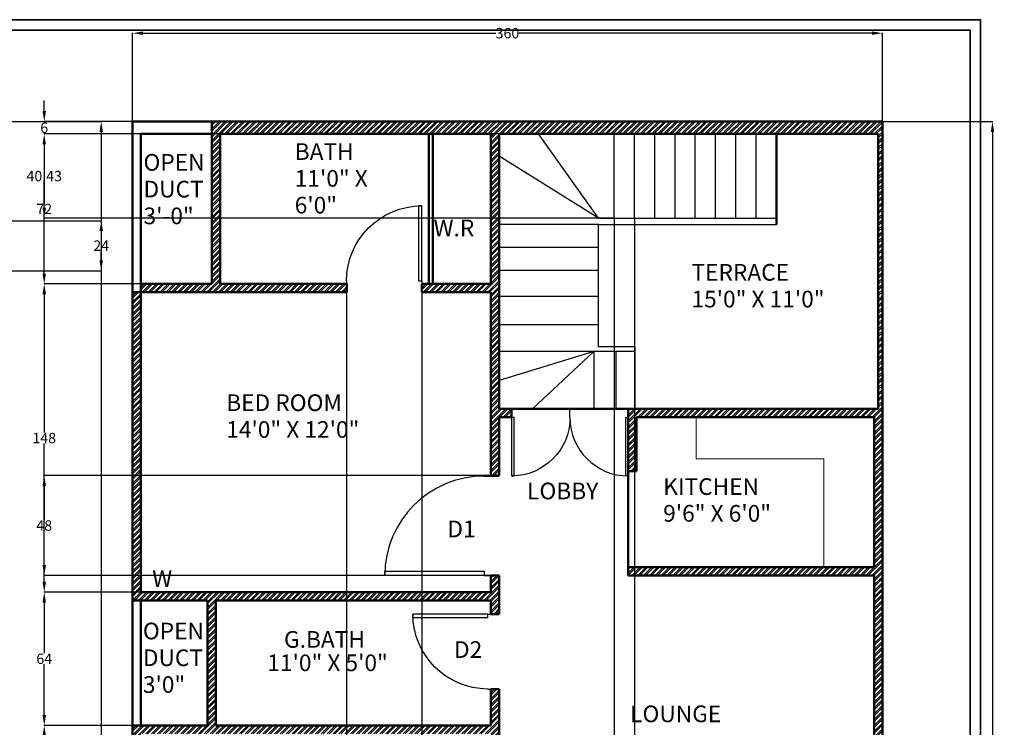
# Model space of a CAD drawing. Units: inches. Extents: x -35 to 905, y -602 to 298.
# Tile 4 of 4: x 429 to 902, y -42 to 298. Entities that reach past the tile are written whole.
import ezdxf

# ---------------------------------------------------------------- set-up
doc = ezdxf.new("R2010")
doc.units = ezdxf.units.IN
doc.header["$MEASUREMENT"] = 0
for name, color, linetype, lineweight in [('A-ANNO-DIMS', 2, 'Continuous', 18), ('A-ANNO-TEXT', 3, 'Continuous', 18), ('A-ANNO-TTLB', 7, 'Continuous', 35), ('A-AREA-IDEN', 7, 'Continuous', 18), ('A-DOOR', 4, 'Continuous', 25), ('A-FLOR-FIXT', 8, 'Continuous', 18), ('A-FLOR-STRS', 3, 'Continuous', 25), ('A-WALL', 7, 'Continuous', 50), ('A-WALL-PATT', 8, 'Continuous', 13)]:
    doc.layers.add(name, color=color, linetype=linetype, lineweight=lineweight)
doc.styles.get("Standard").update_dxf_attribs({"font": 'arial.ttf'})
doc.dimstyles.get("Standard").update_dxf_attribs({"dimtxt": 5, "dimasz": 5, "dimexe": 0.18, "dimexo": 0.0625, "dimgap": 0.09, "dimtad": 0, "dimtih": 1, "dimtoh": 1, "dimdec": 1, "dimzin": 0, "dimdsep": 46, "dimlunit": 4, "dimtxsty": 'Standard', "dimcen": 0.09, "dimadec": 0, "dimazin": 0, "dimtfac": 1, "dimtdec": 1, "dimtofl": 0, "dimtmove": 0, "dimatfit": 3, "dimfxl": 1, "dimtolj": 1, "dimtzin": 0, "dimarcsym": 0})

# ---------------------------------------------------------------- blocks, each defined once
blk = doc.blocks.new('*U2')
for p, q in [((0, 0), (0, -6)), ((40, 0), (40, -6))]:
    blk.add_line(p, q)
blk.add_lwpolyline([(0, 0), (0, 40), (1.75, 40), (1.75, 0)], close=True)
blk.add_arc((0, 0), 40, 0, 90)
blk = doc.blocks.new('*D18')
at = {"layer": 'A-ANNO-DIMS', "color": 0, "lineweight": -2, "ltscale": 0.3, "transparency": 16777216}
for p, q in [((377.85, 249.35), (468.36, 249.35)), ((468.18, 244.35), (468.18, -104.51)), ((468.18, -458.65), (468.18, -109.8)), ((377.85, -463.65), (468.36, -463.65))]:
    blk.add_line(p, q, dxfattribs=at)
at = {"layer": 'A-ANNO-DIMS', "color": 0, "ltscale": 0.3, "transparency": 16777216}
for points in [[(467.35, 244.35), (469.02, 244.35), (468.18, 249.35)], [(467.35, -458.65), (469.02, -458.65), (468.18, -463.65)]]:
    blk.add_solid(points, dxfattribs=at)
at = {"layer": 'Defpoints', "color": 0, "ltscale": 0.3, "transparency": 16777216}
for p in [(377.78, 249.35), (377.78, -463.65), (468.18, -463.65)]:
    blk.add_point(p, dxfattribs=at)
at = {"layer": 'A-ANNO-DIMS', "color": 0, "ltscale": 0.3, "transparency": 16777216, "insert": (468.18, -107.15), "char_height": 5, "attachment_point": 5}
blk.add_mtext('\\A1;713', dxfattribs=at)
blk = doc.blocks.new('*D23')
at = {"layer": 'A-ANNO-DIMS', "color": 0, "lineweight": -2, "ltscale": 0.3, "transparency": 16777216}
for p, q in [((101.85, 201.71), (468.36, 201.71)), ((468.18, 196.71), (468.18, 192.31)), ((468.18, 182.71), (468.18, 187.11)), ((101.85, 177.71), (468.36, 177.71))]:
    blk.add_line(p, q, dxfattribs=at)
at = {"layer": 'A-ANNO-DIMS', "color": 0, "ltscale": 0.3, "transparency": 16777216}
for points in [[(467.35, 196.71), (469.02, 196.71), (468.18, 201.71)], [(467.35, 182.71), (469.02, 182.71), (468.18, 177.71)]]:
    blk.add_solid(points, dxfattribs=at)
at = {"layer": 'Defpoints', "color": 0, "ltscale": 0.3, "transparency": 16777216}
for p in [(101.78, 201.71), (468.18, 201.71), (101.78, 177.71)]:
    blk.add_point(p, dxfattribs=at)
at = {"layer": 'A-ANNO-DIMS', "color": 0, "ltscale": 0.3, "transparency": 16777216, "insert": (468.18, 189.71), "char_height": 5, "attachment_point": 5}
blk.add_mtext('\\A1;24', dxfattribs=at)
blk = doc.blocks.new('*D31')
at = {"layer": 'A-ANNO-DIMS', "color": 0, "lineweight": -2, "ltscale": 0.3, "transparency": 16777216}
for p, q in [((483.24, 249.41), (483.24, 291.93)), ((488.24, 291.75), (657.64, 291.75)), ((838.24, 291.75), (668.84, 291.75)), ((843.24, 249.41), (843.24, 291.93))]:
    blk.add_line(p, q, dxfattribs=at)
at = {"layer": 'A-ANNO-DIMS', "color": 0, "ltscale": 0.3, "transparency": 16777216}
for points in [[(488.24, 292.58), (488.24, 290.91), (483.24, 291.75)], [(838.24, 292.58), (838.24, 290.91), (843.24, 291.75)]]:
    blk.add_solid(points, dxfattribs=at)
at = {"layer": 'Defpoints', "color": 0, "ltscale": 0.3, "transparency": 16777216}
for p in [(843.24, 291.75), (483.24, 249.35), (843.24, 249.35)]:
    blk.add_point(p, dxfattribs=at)
at = {"layer": 'A-ANNO-DIMS', "color": 0, "ltscale": 0.3, "transparency": 16777216, "insert": (663.24, 291.75), "char_height": 5, "attachment_point": 5}
blk.add_mtext('\\A1;360', dxfattribs=at)
blk = doc.blocks.new('*D32')
at = {"layer": 'A-ANNO-DIMS', "color": 0, "lineweight": -2, "ltscale": 0.3, "transparency": 16777216}
for p, q in [((440.84, 254.35), (440.84, 259.35)), ((483.18, 249.35), (440.66, 249.35)), ((487.18, 243.35), (440.66, 243.35)), ((440.84, 238.35), (440.84, 233.35))]:
    blk.add_line(p, q, dxfattribs=at)
at = {"layer": 'A-ANNO-DIMS', "color": 0, "ltscale": 0.3, "transparency": 16777216}
for points in [[(440.01, 254.35), (441.67, 254.35), (440.84, 249.35)], [(440.01, 238.35), (441.67, 238.35), (440.84, 243.35)]]:
    blk.add_solid(points, dxfattribs=at)
at = {"layer": 'Defpoints', "color": 0, "ltscale": 0.3, "transparency": 16777216}
for p in [(483.24, 249.35), (440.84, 243.35), (487.24, 243.35)]:
    blk.add_point(p, dxfattribs=at)
at = {"layer": 'A-ANNO-DIMS', "color": 0, "ltscale": 0.3, "transparency": 16777216, "insert": (440.84, 246.35), "char_height": 5, "attachment_point": 5}
blk.add_mtext('\\A1;6', dxfattribs=at)
blk = doc.blocks.new('*D33')
at = {"layer": 'A-ANNO-DIMS', "color": 0, "lineweight": -2, "ltscale": 0.3, "transparency": 16777216}
for p, q in [((487.18, 243.35), (440.66, 243.35)), ((440.84, 238.35), (440.84, 209.95)), ((440.84, 176.35), (440.84, 204.75)), ((487.18, 171.35), (440.66, 171.35))]:
    blk.add_line(p, q, dxfattribs=at)
at = {"layer": 'A-ANNO-DIMS', "color": 0, "ltscale": 0.3, "transparency": 16777216}
for points in [[(440.01, 238.35), (441.67, 238.35), (440.84, 243.35)], [(440.01, 176.35), (441.67, 176.35), (440.84, 171.35)]]:
    blk.add_solid(points, dxfattribs=at)
at = {"layer": 'Defpoints', "color": 0, "ltscale": 0.3, "transparency": 16777216}
for p in [(487.24, 243.35), (440.84, 171.35), (487.24, 171.35)]:
    blk.add_point(p, dxfattribs=at)
at = {"layer": 'A-ANNO-DIMS', "color": 0, "ltscale": 0.3, "transparency": 16777216, "insert": (440.84, 207.35), "char_height": 5, "attachment_point": 5}
blk.add_mtext('\\A1;72', dxfattribs=at)
blk = doc.blocks.new('*D34')
at = {"layer": 'A-ANNO-DIMS', "color": 0, "lineweight": -2, "ltscale": 0.3, "transparency": 16777216}
for p, q in [((487.18, 171.35), (440.66, 171.35)), ((440.84, 166.35), (440.84, 99.99)), ((440.84, 28.35), (440.84, 94.7)), ((487.18, 23.35), (440.66, 23.35))]:
    blk.add_line(p, q, dxfattribs=at)
at = {"layer": 'A-ANNO-DIMS', "color": 0, "ltscale": 0.3, "transparency": 16777216}
for points in [[(440.01, 166.35), (441.67, 166.35), (440.84, 171.35)], [(440.01, 28.35), (441.67, 28.35), (440.84, 23.35)]]:
    blk.add_solid(points, dxfattribs=at)
at = {"layer": 'Defpoints', "color": 0, "ltscale": 0.3, "transparency": 16777216}
for p in [(487.24, 171.35), (440.84, 23.35), (487.24, 23.35)]:
    blk.add_point(p, dxfattribs=at)
at = {"layer": 'A-ANNO-DIMS', "color": 0, "ltscale": 0.3, "transparency": 16777216, "insert": (440.84, 97.35), "char_height": 5, "attachment_point": 5}
blk.add_mtext('\\A1;148', dxfattribs=at)
blk = doc.blocks.new('*D35')
at = {"layer": 'A-ANNO-DIMS', "color": 0, "lineweight": -2, "ltscale": 0.3, "transparency": 16777216}
for p, q in [((487.18, 23.35), (440.66, 23.35)), ((440.84, 18.35), (440.84, -6.01)), ((440.84, -35.65), (440.84, -11.3)), ((487.18, -40.65), (440.66, -40.65))]:
    blk.add_line(p, q, dxfattribs=at)
at = {"layer": 'A-ANNO-DIMS', "color": 0, "ltscale": 0.3, "transparency": 16777216}
for points in [[(440.01, 18.35), (441.67, 18.35), (440.84, 23.35)], [(440.01, -35.65), (441.67, -35.65), (440.84, -40.65)]]:
    blk.add_solid(points, dxfattribs=at)
at = {"layer": 'Defpoints', "color": 0, "ltscale": 0.3, "transparency": 16777216}
for p in [(487.24, 23.35), (440.84, -40.65), (487.24, -40.65)]:
    blk.add_point(p, dxfattribs=at)
at = {"layer": 'A-ANNO-DIMS', "color": 0, "ltscale": 0.3, "transparency": 16777216, "insert": (440.84, -8.65), "char_height": 5, "attachment_point": 5}
blk.add_mtext('\\A1;64', dxfattribs=at)
blk = doc.blocks.new('*D36')
at = {"layer": 'A-ANNO-DIMS', "color": 0, "lineweight": -2, "ltscale": 0.3, "transparency": 16777216}
for p, q in [((487.18, -40.65), (440.66, -40.65)), ((440.84, -45.65), (440.84, -112.01)), ((440.84, -183.65), (440.84, -117.3)), ((487.18, -188.65), (440.66, -188.65))]:
    blk.add_line(p, q, dxfattribs=at)
at = {"layer": 'A-ANNO-DIMS', "color": 0, "ltscale": 0.3, "transparency": 16777216}
for points in [[(440.01, -45.65), (441.67, -45.65), (440.84, -40.65)], [(440.01, -183.65), (441.67, -183.65), (440.84, -188.65)]]:
    blk.add_solid(points, dxfattribs=at)
at = {"layer": 'Defpoints', "color": 0, "ltscale": 0.3, "transparency": 16777216}
for p in [(487.24, -40.65), (440.84, -188.65), (487.24, -188.65)]:
    blk.add_point(p, dxfattribs=at)
at = {"layer": 'A-ANNO-DIMS', "color": 0, "ltscale": 0.3, "transparency": 16777216, "insert": (440.84, -114.65), "char_height": 5, "attachment_point": 5}
blk.add_mtext('\\A1;148', dxfattribs=at)
blk = doc.blocks.new('*D40')
at = {"layer": 'A-ANNO-DIMS', "color": 0, "lineweight": -2, "ltscale": 0.3, "transparency": 16777216}
for p, q in [((843.3, 249.35), (896.28, 249.35)), ((896.1, 244.35), (896.1, -104.51)), ((896.1, -458.65), (896.1, -109.8)), ((843.3, -463.65), (896.28, -463.65))]:
    blk.add_line(p, q, dxfattribs=at)
at = {"layer": 'A-ANNO-DIMS', "color": 0, "ltscale": 0.3, "transparency": 16777216}
for points in [[(895.27, 244.35), (896.94, 244.35), (896.1, 249.35)], [(895.27, -458.65), (896.94, -458.65), (896.1, -463.65)]]:
    blk.add_solid(points, dxfattribs=at)
at = {"layer": 'Defpoints', "color": 0, "ltscale": 0.3, "transparency": 16777216}
for p in [(843.24, 249.35), (843.24, -463.65), (896.1, -463.65)]:
    blk.add_point(p, dxfattribs=at)
at = {"layer": 'A-ANNO-DIMS', "color": 0, "ltscale": 0.3, "transparency": 16777216, "insert": (896.1, -107.15), "char_height": 5, "attachment_point": 5}
blk.add_mtext('\\A1;713', dxfattribs=at)
blk = doc.blocks.new('*D48')
at = {"layer": 'A-ANNO-DIMS', "color": 0, "lineweight": -2, "ltscale": 0.3, "transparency": 16777216}
for p, q in [((585.99, 167.28), (585.99, -506.23)), ((622.06, 167.28), (622.06, -506.23)), ((590.99, -506.05), (593.54, -506.05)), ((617.06, -506.05), (614.51, -506.05))]:
    blk.add_line(p, q, dxfattribs=at)
at = {"layer": 'A-ANNO-DIMS', "color": 0, "ltscale": 0.3, "transparency": 16777216}
for points in [[(590.99, -505.22), (590.99, -506.89), (585.99, -506.05)], [(617.06, -505.22), (617.06, -506.89), (622.06, -506.05)]]:
    blk.add_solid(points, dxfattribs=at)
at = {"layer": 'Defpoints', "color": 0, "ltscale": 0.3, "transparency": 16777216}
for p in [(585.99, 167.35), (622.06, 167.35), (622.06, -506.05)]:
    blk.add_point(p, dxfattribs=at)
at = {"layer": 'A-ANNO-DIMS', "color": 0, "ltscale": 0.3, "transparency": 16777216, "insert": (604.02, -506.05), "char_height": 5, "attachment_point": 5}
blk.add_mtext('\\A1;36.065', dxfattribs=at)
blk = doc.blocks.new('*D51')
at = {"layer": 'A-ANNO-DIMS', "color": 0, "lineweight": -2, "ltscale": 0.3, "transparency": 16777216}
for p, q in [((655.18, 79.35), (440.66, 79.35)), ((440.84, 74.35), (440.84, 57.99)), ((440.84, 36.35), (440.84, 52.7)), ((655.18, 31.35), (440.66, 31.35))]:
    blk.add_line(p, q, dxfattribs=at)
at = {"layer": 'A-ANNO-DIMS', "color": 0, "ltscale": 0.3, "transparency": 16777216}
for points in [[(440.01, 74.35), (441.67, 74.35), (440.84, 79.35)], [(440.01, 36.35), (441.67, 36.35), (440.84, 31.35)]]:
    blk.add_solid(points, dxfattribs=at)
at = {"layer": 'Defpoints', "color": 0, "ltscale": 0.3, "transparency": 16777216}
for p in [(440.84, 79.35), (655.24, 79.35), (655.24, 31.35)]:
    blk.add_point(p, dxfattribs=at)
at = {"layer": 'A-ANNO-DIMS', "color": 0, "ltscale": 0.3, "transparency": 16777216, "insert": (440.84, 55.35), "char_height": 5, "attachment_point": 5}
blk.add_mtext('\\A1;48', dxfattribs=at)
blk = doc.blocks.new('*D52')
at = {"layer": 'A-ANNO-DIMS', "color": 0, "lineweight": -2, "ltscale": 0.3, "transparency": 16777216}
for p, q in [((714.42, 202.86), (714.42, -506.23)), ((724.17, 202.86), (724.17, -506.23)), ((709.42, -506.05), (704.42, -506.05)), ((729.17, -506.05), (734.17, -506.05))]:
    blk.add_line(p, q, dxfattribs=at)
at = {"layer": 'A-ANNO-DIMS', "color": 0, "ltscale": 0.3, "transparency": 16777216}
for points in [[(709.42, -505.22), (709.42, -506.89), (714.42, -506.05)], [(729.17, -505.22), (729.17, -506.89), (724.17, -506.05)]]:
    blk.add_solid(points, dxfattribs=at)
at = {"layer": 'Defpoints', "color": 0, "ltscale": 0.3, "transparency": 16777216}
for p in [(714.42, 202.92), (724.17, 202.92), (724.17, -506.05)]:
    blk.add_point(p, dxfattribs=at)
at = {"layer": 'A-ANNO-DIMS', "color": 0, "ltscale": 0.3, "transparency": 16777216, "insert": (742.7, -506.05), "char_height": 5, "attachment_point": 5}
blk.add_mtext('\\A1;9.753', dxfattribs=at)
blk = doc.blocks.new('*D53')
at = {"layer": 'A-ANNO-DIMS', "color": 0, "lineweight": -2, "ltscale": 0.3, "transparency": 16777216}
for p, q in [((714.36, 243.35), (440.66, 243.35)), ((440.84, 238.35), (440.84, 225.78)), ((440.84, 207.92), (440.84, 220.49)), ((714.36, 202.92), (440.66, 202.92))]:
    blk.add_line(p, q, dxfattribs=at)
at = {"layer": 'A-ANNO-DIMS', "color": 0, "ltscale": 0.3, "transparency": 16777216}
for points in [[(440.01, 238.35), (441.67, 238.35), (440.84, 243.35)], [(440.01, 207.92), (441.67, 207.92), (440.84, 202.92)]]:
    blk.add_solid(points, dxfattribs=at)
at = {"layer": 'Defpoints', "color": 0, "ltscale": 0.3, "transparency": 16777216}
for p in [(714.42, 243.35), (440.84, 202.92), (714.42, 202.92)]:
    blk.add_point(p, dxfattribs=at)
at = {"layer": 'A-ANNO-DIMS', "color": 0, "ltscale": 0.3, "transparency": 16777216, "insert": (440.84, 223.13), "char_height": 5, "attachment_point": 5}
blk.add_mtext('\\A1;40.43', dxfattribs=at)

msp = doc.modelspace()

# ---------------------------------------------------------------- hatches: boundary and pattern name
at = {"layer": 'A-WALL-PATT', "ltscale": 0.3}
h = msp.add_hatch(dxfattribs=at)
h.set_pattern_fill('ANSI32', color=256, scale=5.3)
h.set_pattern_definition([(45, (-58.8752, 0), (-1.4053747, 1.4053747), []), (45, (-57.9383, 0), (-1.4053747, 1.4053747), [])])
h.paths.add_polyline_path([(843.2385, 107.3466), (843.2385, 249.3466), (521.2385, 249.3466), (521.2385, 171.3466), (487.2385, 171.3466), (487.2385, 167.3466), (586.0557, 167.3466), (586.0557, 171.3466), (567.2385, 171.3466), (525.2385, 171.3466), (525.2385, 243.3466), (571.2385, 243.3466), (655.2385, 243.3466), (655.2385, 213.7106), (655.2385, 171.3466), (622.0557, 171.3466), (622.0557, 167.3466), (655.2385, 167.3466), (655.2385, 79.3466), (659.2385, 79.3466), (659.2385, 107.3466), (665.2408, 107.3466), (665.2408, 111.3466), (659.2385, 111.3466), (659.2385, 213.7106), (659.2385, 243.3466), (841.2385, 243.3466), (841.2385, 111.3466), (721.2578, 111.3466), (721.2578, 107.1453), (721.2578, 81.4115), (725.2385, 81.4115), (725.2385, 107.3466), (839.2385, 107.3466), (839.2385, 35.3466), (721.2385, 35.3466), (721.2385, 31.3466), (839.2385, 31.3466), (839.2385, -160.6534), (713.2385, -160.6534), (713.2385, -164.6534), (713.2385, -212.6534), (717.2385, -212.6534), (717.2385, -164.6534), (843.2385, -164.6534), (849.7023, -164.6534), (849.7023, -260.6534), (843.2385, -260.6534), (843.2385, -264.6534), (853.7023, -264.6534), (853.7023, -160.6534), (843.2385, -160.6534)])
h.paths.add_polyline_path([(655.2385, -188.6534), (655.2385, -192.6534), (659.2385, -192.6534), (659.2385, -23.1851), (655.2385, -23.1851), (655.2385, -40.6534), (523.2385, -40.6534), (523.2385, 19.3466), (655.2385, 19.3466), (655.2385, 12.8149), (659.2385, 12.8149), (659.2385, 31.3466), (655.2385, 31.3466), (655.2385, 23.3466), (487.2385, 23.3466), (487.2385, 167.3466), (483.2385, 167.3466), (483.2385, 19.3466), (519.2385, 19.3466), (519.2385, -40.6534), (483.2385, -40.6534), (483.2385, -463.6534), (487.2385, -463.6534), (487.2385, -422.6534), (496.4926, -422.6534), (496.4926, -422.2505), (496.4926, -418.6534), (487.2385, -418.6534), (487.2385, -315.6534), (487.2385, -192.6534), (487.2385, -44.6534), (655.2385, -44.6534)])
h.paths.add_polyline_path([(523.2385, -315.6534), (568.9907, -315.6534), (568.9907, -311.6534), (527.2385, -311.6534), (527.2385, -254.1534), (608.2385, -254.1534), (608.2385, -311.6534), (604.9907, -311.6534), (604.9907, -315.6534), (612.2385, -315.6534), (612.2385, -250.1534), (612.2385, -188.6534), (604.9907, -188.6534), (604.9907, -192.6534), (608.2385, -192.6534), (608.2385, -250.1534), (527.2385, -250.1534), (527.2385, -192.6534), (568.8266, -192.6534), (568.8266, -188.6534), (523.2385, -188.6534)], flags=17)
h.paths.add_polyline_path([(655.2385, -313.832), (655.2385, -418.6534), (520.4926, -418.6534), (520.4926, -422.6534), (655.2385, -422.6534), (655.2385, -461.6534), (655.2385, -463.6534), (659.2385, -463.6534), (659.2385, -457.6052), (659.2385, -422.6534), (664.6743, -422.6534), (664.6743, -422.2478), (664.6743, -418.6534), (659.2385, -418.6534), (659.2385, -311.6534), (669.6291, -302.6097), (667.0409, -299.5595), (655.2385, -309.832), (649.2787, -309.832), (649.2787, -313.832)])
h.paths.add_polyline_path([(839.2385, -264.6534), (839.2385, -407.6534), (836.0142, -407.6534), (836.0142, -411.6534), (839.2385, -411.6534), (839.2385, -459.6534), (767.2385, -459.6534), (767.2385, -411.6534), (800.0142, -411.6534), (800.0142, -407.6534), (767.2385, -407.6534), (763.2385, -407.6534), (763.2385, -418.6534), (688.6743, -418.6534), (688.6743, -422.6534), (763.2385, -422.6534), (763.2385, -463.6534), (843.2385, -463.6534), (843.2385, -260.6534), (715.7415, -260.6534), (715.7415, -251.2468), (711.7415, -251.2468), (711.7415, -260.6534), (704.4179, -267.0277), (702.7449, -268.4838), (705.371, -271.5011), (707.044, -270.0449), (713.2385, -264.6534)])
h.paths.add_polyline_path([(592.7587, -420.6534), (607.3071, -420.6534), (607.3071, -408.6534), (592.7587, -408.6534)], flags=24)
h.paths.add_polyline_path([(723.9564, -420.6534), (738.5048, -420.6534), (738.5048, -408.6534), (723.9564, -408.6534)], flags=24)

# ---------------------------------------------------------------- linework, layer by layer
at = {"layer": 'A-ANNO-TTLB', "ltscale": 0.3}
for points in [[(-16.7606, 298.2205), (890.3824, 298.2205), (890.3824, -602.0527), (-16.7606, -602.0527)], [(-11.7606, 293.2205), (885.3824, 293.2205), (885.3824, -599.6301), (-11.7606, -599.6301)]]:
    msp.add_lwpolyline(points, close=True, dxfattribs=at)
at = {"layer": 'A-FLOR-FIXT', "ltscale": 0.3}
for p, q in [((753.8854, 87.3211), (753.8854, 107.3466)), ((815.1608, 87.3211), (753.8854, 87.3211)), ((815.1608, 81.4115), (815.1608, 87.3211))]:
    msp.add_line(p, q, dxfattribs=at)
at = {"layer": 'A-FLOR-FIXT'}
msp.add_line((815.1608, 81.4115), (815.1608, 35.3466), dxfattribs=at)
at = {"layer": 'A-FLOR-STRS', "ltscale": 0.3}
for p, q in [((706.8936, 202.9184), (678.1479, 243.3466)), ((714.4218, 202.9184), (714.4218, 243.3466)), ((724.1748, 202.9184), (724.1748, 243.3466)), ((733.9277, 202.9184), (733.9277, 243.3466)), ((743.6806, 202.9184), (743.6806, 243.3466)), ((753.4336, 202.9184), (753.4336, 243.3466)), ((763.1865, 202.9184), (763.1865, 243.3466)), ((772.9394, 202.9184), (772.9394, 243.3466)), ((782.6924, 202.9184), (782.6924, 243.3466)), ((706.8936, 202.9184), (659.2385, 232.7531)), ((706.8936, 199.9184), (659.2385, 199.9184)), ((706.8936, 202.9184), (792.4453, 202.9184)), ((706.8936, 141.0839), (706.8936, 199.9184)), ((706.8936, 199.9184), (792.4453, 199.9184)), ((706.8936, 188.8347), (659.2385, 188.8347)), ((706.8936, 177.8594), (659.2385, 177.8594)), ((706.8936, 165.2442), (659.2385, 165.2442)), ((706.8936, 151.7806), (659.2385, 151.7806)), ((724.4958, 138.8376), (659.2385, 138.8376)), ((704.7572, 138.8376), (659.2385, 124.9608)), ((704.7572, 138.8376), (675.2188, 111.3466)), ((704.7572, 138.8376), (704.7572, 111.3466)), ((724.4958, 141.0839), (706.8936, 141.0839)), ((715.2345, 138.8376), (715.2345, 111.3466)), ((724.4958, 111.3466), (724.4958, 141.0839)), ((721.2385, 111.3466), (724.4958, 111.3466))]:
    msp.add_line(p, q, dxfattribs=at)
at = {"layer": 'A-WALL'}
for p, q in [((483.2385, 249.3466), (483.2385, -463.6534)), ((483.2385, 249.3466), (843.2385, 249.3466)), ((521.2385, 249.3466), (521.2385, 171.3466)), ((843.2385, 249.3466), (843.2385, 107.3466)), ((487.2385, 243.3466), (487.2385, 167.3466)), ((487.2385, 243.3466), (521.2385, 243.3466)), ((525.2385, 243.3466), (525.2385, 171.3466)), ((525.2385, 243.3466), (571.2385, 243.3466)), ((571.2385, 243.3466), (655.2385, 243.3466)), ((625.4546, 243.3466), (625.4546, 171.3466)), ((627.4445, 243.3466), (627.4445, 171.3466)), ((655.2385, 243.3466), (655.2385, 213.7106)), ((659.2385, 243.3466), (659.2385, 213.7106)), ((659.2385, 243.3466), (841.2385, 243.3466)), ((841.2385, 243.3466), (841.2385, 111.3466)), ((655.2385, 213.7106), (655.2385, 171.3466)), ((659.2385, 213.7106), (659.2385, 111.3466)), ((487.2385, 171.3466), (521.2385, 171.3466)), ((525.2385, 171.3466), (567.2385, 171.3466)), ((567.2385, 171.3466), (586.0557, 171.3466)), ((622.0557, 171.3466), (655.2385, 171.3466)), ((483.2385, 167.3466), (586.0557, 167.3466)), ((487.2385, 167.3466), (487.2385, 23.3466)), ((622.0557, 167.3466), (655.2385, 167.3466)), ((655.2385, 167.3466), (655.2385, 79.3466)), ((659.2385, 111.3466), (665.2408, 111.3466)), ((665.2408, 111.3466), (665.2408, 107.3466)), ((721.2385, 111.3466), (721.2385, 81.4115)), ((721.2385, 111.3466), (841.2385, 111.3466)), ((659.2385, 107.3466), (659.2385, 79.3466)), ((659.2385, 107.3466), (665.2408, 107.3466)), ((725.2385, 107.3466), (725.2385, 81.4115)), ((725.2385, 107.3466), (839.2385, 107.3466)), ((839.2385, 107.3466), (839.2385, 35.3466)), ((843.2385, 107.3466), (843.2385, -160.6534)), ((721.2385, 81.4115), (725.2385, 81.4115)), ((655.2385, 79.3466), (659.2385, 79.3466)), ((721.2385, 35.3466), (721.2385, 31.3466)), ((721.2385, 35.3466), (839.2385, 35.3466)), ((655.2385, 31.3466), (655.2385, 23.3466)), ((659.2385, 31.3466), (655.2385, 31.3466)), ((659.2385, 31.3466), (659.2385, 12.8149)), ((721.2385, 31.3466), (839.2385, 31.3466)), ((839.2385, 31.3466), (839.2385, -160.6534)), ((483.2385, 19.3466), (519.2385, 19.3466)), ((487.2385, 23.3466), (655.2385, 23.3466)), ((487.2385, 19.3466), (487.2385, -40.6534)), ((519.2385, 19.3466), (519.2385, -40.6534)), ((523.2385, 19.3466), (523.2385, -40.6534)), ((523.2385, 19.3466), (655.2385, 19.3466)), ((655.2385, 19.3466), (655.2385, 12.8149)), ((655.2385, -23.1851), (655.2385, -40.6534)), ((659.2385, -23.1851), (659.2385, -192.6534)), ((483.2385, -40.6534), (519.2385, -40.6534)), ((523.2385, -40.6534), (655.2385, -40.6534))]:
    msp.add_line(p, q, dxfattribs=at)
at = {"layer": 'A-WALL', "ltscale": 0.3}
for p, q in [((792.4453, 199.9184), (792.4453, 243.3466)), ((792.4453, 202.9184), (792.4453, 243.3466)), ((586.0557, 167.3466), (586.0557, 171.3466)), ((622.0557, 171.3466), (622.0557, 167.3466)), ((665.2408, 111.3466), (721.2385, 111.3466)), ((721.2385, 81.4115), (721.2385, 35.3466)), ((655.2385, 12.8149), (659.2385, 12.8149)), ((659.2385, -23.1851), (655.2385, -23.1851))]:
    msp.add_line(p, q, dxfattribs=at)

# ---------------------------------------------------------------- block references
at = {"layer": 'A-DOOR', "xscale": -0.9016333179236413, "yscale": 0.9016333179236413, "zscale": 0.9016333179236413}
msp.add_blockref('*U2', (622.0557, 172.7564), dxfattribs=at)
at = {"layer": 'A-DOOR'}
for p, xscale, yscale, zscale, rotation in [((665.2408, 107.1453), -0.700211784135817, 0.700211784135817, 0.700211784135817, 180), ((721.2578, 107.1453), 0.700211784135817, 0.700211784135817, 0.700211784135817, 180), ((652.0788, 31.3466), 1.193272600612834, 1.193272600612834, 1.193272600612834, 90), ((653.8405, 12.8149), -0.8996531203609501, 0.8996531203609501, 0.8996531203609501, 90)]:
    msp.add_blockref('*U2', p, dxfattribs=dict(at, xscale=xscale, yscale=yscale, zscale=zscale, rotation=rotation))

# ---------------------------------------------------------------- texts
at = {"layer": 'A-ANNO-TEXT', "ltscale": 0.3}
for s, p in [('D1', (634.3997, 49.6984)), ('W', (492.6738, 25.8812)), ('D2', (637.5688, -8.2236))]:
    msp.add_text(s, height=8, dxfattribs=at).set_placement(p)
at = {"layer": 'A-AREA-IDEN', "ltscale": 0.3}
for s, p in [('BATH', (561.0987, 230.8827)), ('OPEN', (488.4988, 225.7201)), ('11\'0" X', (561.0987, 218.0315)), ('DUCT', (488.4988, 212.8688)), ('6\'0"', (561.0987, 205.1802)), ('3\'-0"', (488.4988, 200.0175)), ('W.R', (627.762, 194.1977)), ('TERRACE', (751.5889, 172.9165)), ('15\'0" X 11\'0"', (751.5889, 160.0652)), ('BED ROOM', (528.2172, 110.3125)), ('14\'0" X 12\'0"', (528.2172, 97.4612)), ('LOBBY', (672.6687, 67.9311)), ('KITCHEN', (738.0031, 70.0342)), ('9\'6" X 6\'0"', (738.0031, 57.1829)), ('OPEN', (488.1998, 0.6878)), ('G.BATH', (555.9427, -3.3444)), ('DUCT', (488.1998, -12.1635)), ('11\'0" X 5\'0"', (547.9479, -14.58)), ('3\'0"', (488.1998, -25.0148)), ('LOUNGE', (722.1408, -39.0929))]:
    msp.add_text(s, height=8, dxfattribs=at).set_placement(p)

# ---------------------------------------------------------------- dimensions: what is measured, and where the dimension line sits
at = {"layer": 'A-ANNO-DIMS', "ltscale": 0.3}
for base, p1, p2, override, picture, middle in [((843.2385, 291.7466), (483.2385, 249.3466), (843.2385, 249.3466), {"dimdec": 0, "dimlfac": 1, "dimrnd": 0, "dimzin": 0, "dimdsep": 46, "dimlunit": 2}, '*D31', (663.2385, 291.7466)), ((724.1748, -506.0534), (714.4218, 202.9184), (724.1748, 202.9184), {"dimdec": 3, "dimlfac": 1, "dimrnd": 0, "dimzin": 0, "dimdsep": 46, "dimlunit": 2}, '*D52', (742.701, -506.0534)), ((622.0557, -506.0534), (585.9904, 167.3466), (622.0557, 167.3466), {"dimdec": 3, "dimlfac": 1, "dimrnd": 0, "dimzin": 0, "dimdsep": 46, "dimlunit": 2}, '*D48', (604.023, -506.0534))]:
    dim = msp.add_linear_dim(base=base, p1=p1, p2=p2, dimstyle='Standard', override=override, dxfattribs=at)
    dim.commit()
    dim.dimension.update_dxf_attribs({"geometry": picture, "text_midpoint": middle})
for base, p1, p2, override, picture, middle in [((440.8385, 243.3466), (483.2385, 249.3466), (487.2385, 243.3466), {"dimdec": 0, "dimlfac": 1, "dimrnd": 0, "dimzin": 0, "dimdsep": 46, "dimlunit": 2}, '*D32', (440.8385, 246.3466)), ((468.1847, -463.6534), (377.7847, 249.3466), (377.7847, -463.6534), {"dimdec": 0, "dimlfac": 1, "dimrnd": 0, "dimzin": 0, "dimdsep": 46, "dimlunit": 2}, '*D18', (468.1847, -107.1534)), ((896.1023, -463.6534), (843.2385, 249.3466), (843.2385, -463.6534), {"dimdec": 0, "dimlfac": 1, "dimrnd": 0, "dimzin": 0, "dimdsep": 46, "dimlunit": 2}, '*D40', (896.1023, -107.1534)), ((440.8385, 202.9184), (714.4218, 243.3466), (714.4218, 202.9184), {"dimdec": 2, "dimlfac": 1, "dimrnd": 0, "dimzin": 0, "dimdsep": 46, "dimlunit": 2}, '*D53', (440.8385, 223.1325)), ((440.8385, 171.3466), (487.2385, 243.3466), (487.2385, 171.3466), {"dimdec": 0, "dimlfac": 1, "dimrnd": 0, "dimzin": 0, "dimdsep": 46, "dimlunit": 2}, '*D33', (440.8385, 207.3466)), ((468.1847, 201.7106), (101.7847, 177.7106), (101.7847, 201.7106), {"dimdec": 0, "dimlfac": 1, "dimrnd": 0, "dimzin": 0, "dimdsep": 46, "dimlunit": 2}, '*D23', (468.1847, 189.7106)), ((440.8385, 23.3466), (487.2385, 171.3466), (487.2385, 23.3466), {"dimdec": 0, "dimlfac": 1, "dimrnd": 0, "dimzin": 0, "dimdsep": 46, "dimlunit": 2}, '*D34', (440.8385, 97.3466)), ((440.8385, 79.3466), (655.2385, 31.3466), (655.2385, 79.3466), {"dimdec": 0, "dimlfac": 1, "dimrnd": 0, "dimzin": 0, "dimdsep": 46, "dimlunit": 2}, '*D51', (440.8385, 55.3466)), ((440.8385, -40.6534), (487.2385, 23.3466), (487.2385, -40.6534), {"dimdec": 0, "dimlfac": 1, "dimrnd": 0, "dimzin": 0, "dimdsep": 46, "dimlunit": 2}, '*D35', (440.8385, -8.6534)), ((440.8385, -188.6534), (487.2385, -40.6534), (487.2385, -188.6534), {"dimdec": 0, "dimlfac": 1, "dimrnd": 0, "dimzin": 0, "dimdsep": 46, "dimlunit": 2}, '*D36', (440.8385, -114.6534))]:
    dim = msp.add_linear_dim(base=base, p1=p1, p2=p2, angle=90, dimstyle='Standard', override=override, dxfattribs=at)
    dim.commit()
    dim.dimension.update_dxf_attribs({"geometry": picture, "text_midpoint": middle})

doc.saveas('drawing.dxf')
